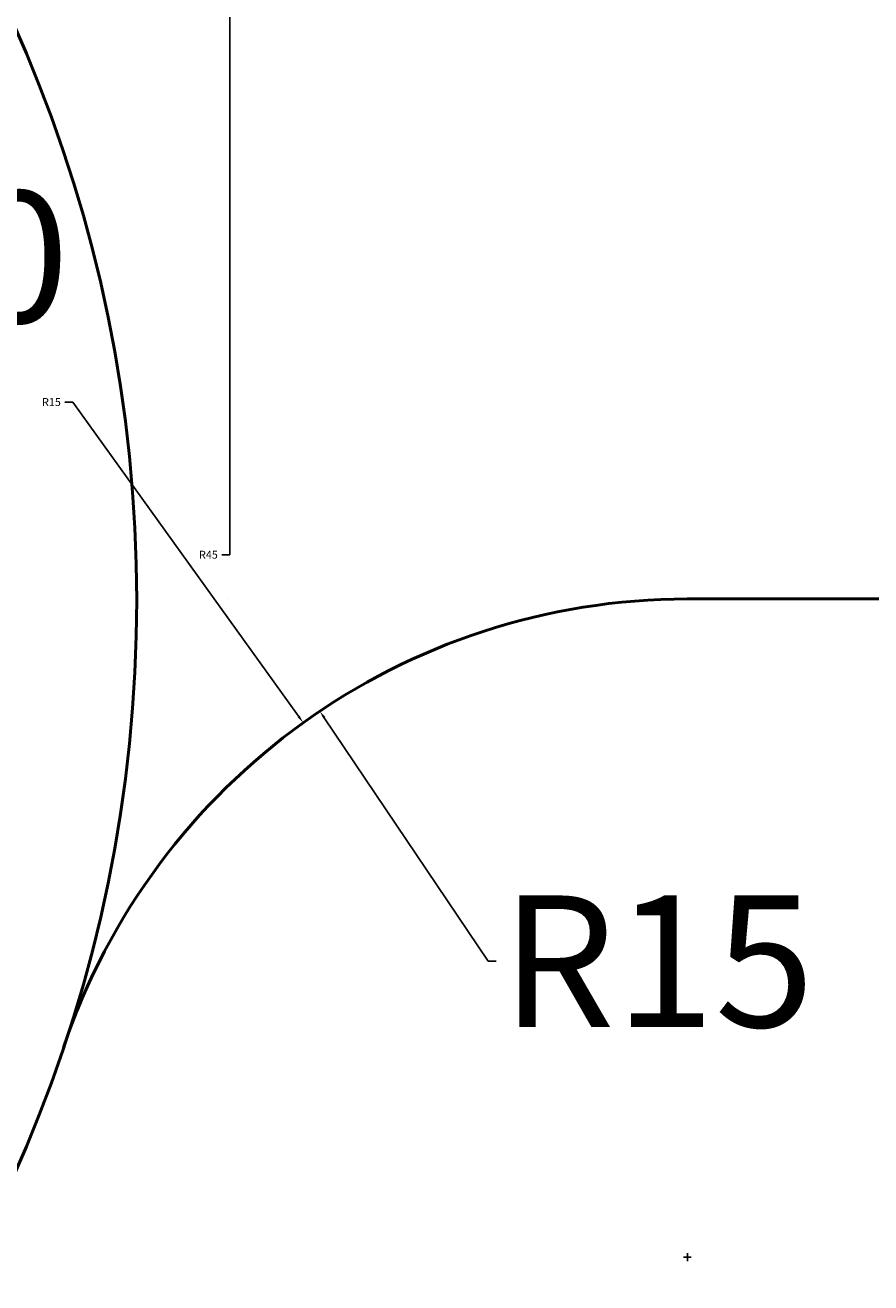
# Model space of a CAD drawing. Units: millimetres. Extents: x -50 to 109, y -46 to 152.
# Tile 7 of 18: x 29 to 48, y -22 to 6. Entities that reach past the tile are written whole.
import ezdxf

# ---------------------------------------------------------------- set-up
doc = ezdxf.new("R2010")
doc.units = ezdxf.units.MM
doc.header["$MEASUREMENT"] = 0
doc.layers.add('M-DIMS', color=2, linetype='Continuous', lineweight=25)
doc.layers.add('M-OUTL', color=7, linetype='Continuous', lineweight=50)
doc.styles.get("Standard").update_dxf_attribs({"font": 'arial.ttf'})
doc.dimstyles.get("Standard").update_dxf_attribs({"dimtxt": 0.18, "dimasz": 0.18, "dimexe": 0.18, "dimexo": 0.0625, "dimgap": 0.09, "dimtad": 0, "dimtih": 1, "dimtoh": 1, "dimdec": 4, "dimzin": 0, "dimdsep": 46, "dimtxsty": 'Standard', "dimcen": 0.09, "dimadec": 0, "dimazin": 0, "dimtfac": 1, "dimtdec": 4, "dimtofl": 0, "dimtmove": 0, "dimatfit": 3, "dimfxl": 1, "dimtolj": 1, "dimtzin": 0, "dimarcsym": 0})

# ---------------------------------------------------------------- blocks, each defined once
blk = doc.blocks.new('*D20')
at = {"layer": 'Defpoints', "color": 0, "transparency": 16777216}
for p in [(21.766, 5.813), (24.805, -3.739), (27.264, -3.739)]:
    blk.add_point(p, dxfattribs=at)
at = {"layer": 'M-DIMS', "color": 0, "lineweight": -2, "transparency": 16777216}
for p, q in [((21.828, 5.813), (27.444, 5.813)), ((27.264, 5.633), (27.264, 2.659)), ((27.264, -3.559), (27.264, -0.585)), ((24.868, -3.739), (27.444, -3.739))]:
    blk.add_line(p, q, dxfattribs=at)
at = {"layer": 'M-DIMS', "color": 0, "transparency": 16777216}
for points in [[(27.234, 5.633), (27.294, 5.633), (27.264, 5.813)], [(27.234, -3.559), (27.294, -3.559), (27.264, -3.739)]]:
    blk.add_solid(points, dxfattribs=at)
at = {"layer": 'M-DIMS', "color": 0, "transparency": 16777216, "insert": (27.264, 1.037), "char_height": 0.18, "attachment_point": 5}
blk.add_mtext('\\A1;{\\H16.66667x;10}', dxfattribs=at)
blk = doc.blocks.new('*D21')
at = {"layer": 'Defpoints', "color": 0, "transparency": 16777216}
for p in [(35.251, -9.315), (43.627, -21.759)]:
    blk.add_point(p, dxfattribs=at)
at = {"layer": 'M-DIMS', "color": 0, "lineweight": -2, "transparency": 16777216}
for p, q in [((39.087, -15.015), (35.351, -9.465)), ((39.267, -15.015), (39.087, -15.015))]:
    blk.add_line(p, q, dxfattribs=at)
at = {"layer": 'M-DIMS', "color": 0, "transparency": 16777216}
blk.add_solid([(35.376, -9.448), (35.326, -9.482), (35.251, -9.315)], dxfattribs=at)
at = {"layer": 'M-DIMS', "color": 0, "transparency": 16777216, "insert": (42.953, -15.015), "char_height": 0.18, "attachment_point": 5}
blk.add_mtext('\\A1;{\\H16.66667x;R15}', dxfattribs=at)
blk = doc.blocks.new('*D33')
at = {"layer": 'Defpoints', "color": 0, "transparency": 16777216}
for p in [(34.872, -9.579), (43.627, -21.759)]:
    blk.add_point(p, dxfattribs=at)
at = {"layer": 'M-DIMS', "color": 0, "lineweight": -2, "transparency": 16777216}
for p, q in [((29.439, -2.271), (29.619, -2.271)), ((29.619, -2.271), (34.767, -9.433)), ((43.537, -21.759), (43.717, -21.759)), ((43.627, -21.849), (43.627, -21.669))]:
    blk.add_line(p, q, dxfattribs=at)
at = {"layer": 'M-DIMS', "color": 0, "transparency": 16777216}
blk.add_solid([(34.791, -9.415), (34.743, -9.45), (34.872, -9.579)], dxfattribs=at)
at = {"layer": 'M-DIMS', "color": 0, "transparency": 16777216, "insert": (29.133, -2.271), "char_height": 0.18, "attachment_point": 5}
blk.add_mtext('\\A1;R15', dxfattribs=at)
blk = doc.blocks.new('*D39')
at = {"layer": 'Defpoints', "color": 0, "transparency": 16777216}
for p in [(33.197, 66.25), (33.197, 21.25)]:
    blk.add_point(p, dxfattribs=at)
at = {"layer": 'M-DIMS', "color": 0, "lineweight": -2, "transparency": 16777216}
for p, q in [((33.107, 66.25), (33.287, 66.25)), ((33.197, 66.16), (33.197, 66.34)), ((33.197, -5.75), (33.197, 21.07)), ((33.017, -5.75), (33.197, -5.75))]:
    blk.add_line(p, q, dxfattribs=at)
at = {"layer": 'M-DIMS', "color": 0, "transparency": 16777216}
blk.add_solid([(33.167, 21.07), (33.227, 21.07), (33.197, 21.25)], dxfattribs=at)
at = {"layer": 'M-DIMS', "color": 0, "transparency": 16777216, "insert": (32.711, -5.75), "char_height": 0.18, "attachment_point": 5}
blk.add_mtext('\\A1;R45', dxfattribs=at)

msp = doc.modelspace()

# ---------------------------------------------------------------- linework, layer by layer
at = {"layer": 'M-OUTL'}
for p, q in [((33.14503, -6.75826), (33.14503, -6.75888)), ((77.14026, -6.75888), (43.62689, -6.75888))]:
    msp.add_line(p, q, dxfattribs=at)
msp.add_circle((-0.92366, -6.78396), 32, dxfattribs=at)
msp.add_arc((43.62689, -21.75888), 15, 90, 161.420799, dxfattribs=at)

# ---------------------------------------------------------------- dimensions: what is measured, and where the dimension line sits
at = {"layer": 'M-DIMS'}
for center, mpoint, picture, middle in [((33.197, 66.24997), (33.197, 21.24997), '*D39', (32.71127, -5.75003)), ((43.62689, -21.75888), (34.87195, -9.57893), '*D33', (29.13326, -2.27097))]:
    dim = msp.add_radius_dim(center=center, mpoint=mpoint, dimstyle='Standard', override={"dimdec": 0, "dimlfac": 1, "dimrnd": 0, "dimzin": 0, "dimdsep": 46, "dimlunit": 2}, dxfattribs=at)
    dim.commit()
    dim.dimension.update_dxf_attribs({"geometry": picture, "text_midpoint": middle, "dimtype": 164})
dim = msp.add_linear_dim(base=(27.26425, -3.73924), p1=(21.76599, 5.81281), p2=(24.80523, -3.73924), angle=90, text='{\\H16.66667x;10}', dimstyle='Standard', override={"dimclrd": 0, "dimclre": 0, "dimclrt": 0}, dxfattribs=at)
dim.commit()
dim.dimension.update_dxf_attribs({"geometry": '*D20', "text_midpoint": (27.26425, 1.03679)})
dim = msp.add_radius_dim(center=(43.62689, -21.75888), mpoint=(35.25066, -9.31545), text='{\\H16.66667x;R15}', dimstyle='Standard', override={"dimclrd": 0, "dimclre": 0, "dimclrt": 0}, dxfattribs=at)
dim.commit()
dim.dimension.update_dxf_attribs({"geometry": '*D21', "text_midpoint": (42.95262, -15.01475), "dimtype": 164})

doc.saveas('drawing.dxf')
